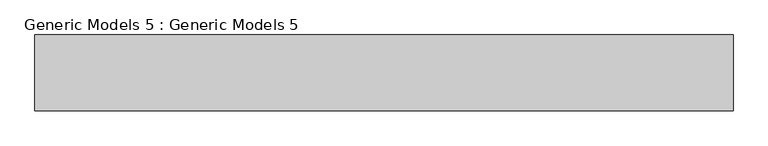
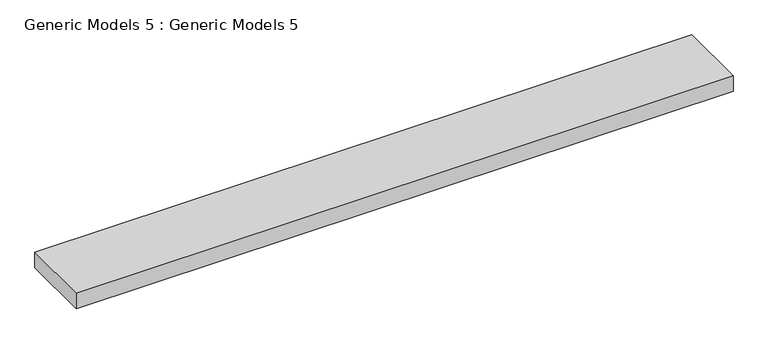
"""IFC4 building model written with IfcOpenShell, lengths in millimetres: proxy geometry, Generic Models 5 : Generic Models 5."""

from ifc_helpers import new_model, si_unit, frame, origin, place, context, project, spatial, polyline, outline, extrude, source, transform, mapped, element, save


def generic_models_5_generic_models_5_1681292e(model_context):
    return source(origin(), model_context, "Body", "SweptSolid", [
        extrude(outline(polyline([(-20359.5457338, -4370.2195077), (-16168.5457338, -4370.2195077), (-16168.5457338, -4826.4776737), (-20359.5457338, -4826.4776737), (-20359.5457338, -4370.2195077)])), frame((0.0, 0.0, 7524.75), z_axis=(0.0, 0.0, 1.0), x_axis=(1.0, 0.0, 0.0)), (0.0, 0.0, 1.0), 103.4551699),
    ])


if __name__ == "__main__":
    model = new_model("IFC4")
    model_context = context("Model", 3, world=origin())
    ifc_project = project(units=[si_unit("LENGTHUNIT", "METRE", prefix="MILLI")], contexts=[model_context])
    site = spatial("IfcSite", under=ifc_project)
    building = spatial("IfcBuilding", under=site)
    placement = place(None, origin())
    generic_models_5_generic_models_5_shape = generic_models_5_generic_models_5_1681292e(model_context)
    element("IfcBuildingElementProxy", 1, Name="Generic Models 5 : Generic Models 5", ObjectType="Generic Models 5 : Generic Models 5", at=placement, inside=building, context=model_context, shape_type="MappedRepresentation", body=[
        mapped(generic_models_5_generic_models_5_shape, transform((0.0, 0.0, 0.0), x_axis=(1.0, 0.0, 0.0), y_axis=(0.0, 1.0, 0.0), z_axis=(0.0, 0.0, 1.0))),
    ])
    save(model, "model.ifc")
